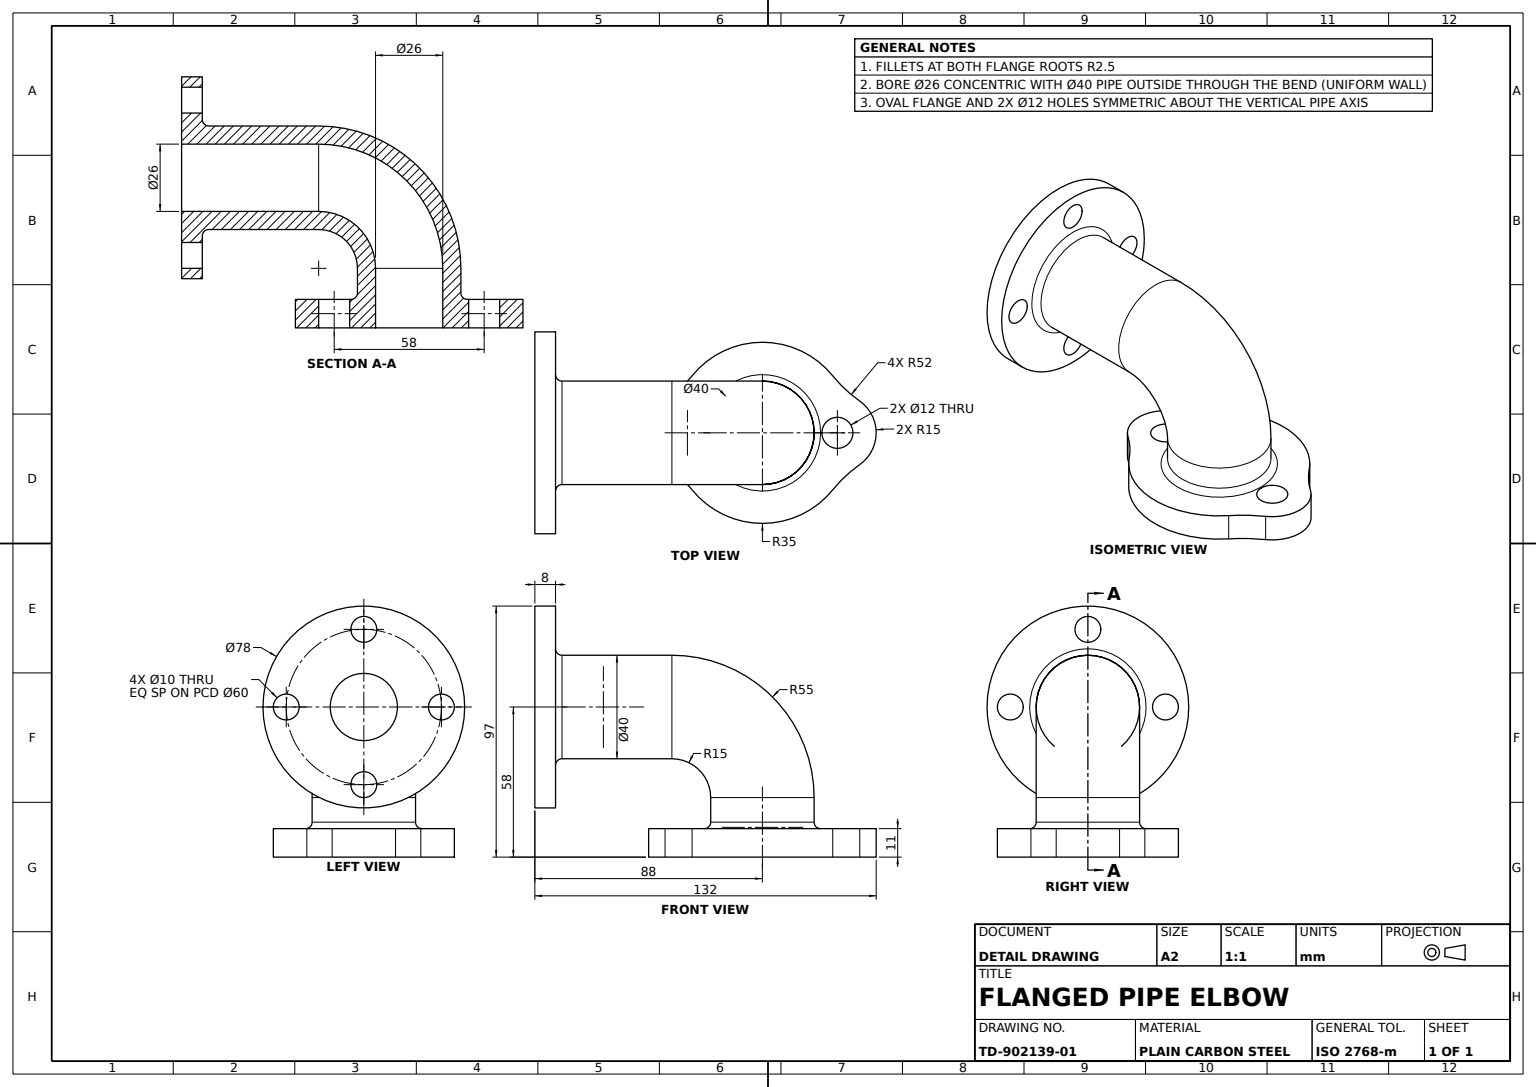
SolidWorks part; units mm, degrees
material "Plain Carbon Steel"
ref_plane "Front Plane" through (0, 0, 0) normal (0, 0, 1) x (1, 0, 0)
ref_plane "Top Plane" through (0, 0, 0) normal (0, 1, 0) x (1, 0, 0)
ref_plane "Right Plane" through (0, 0, 0) normal (1, 0, 0) x (0, 0, -1)
sketch "Elbow Path Sketch" plane through (0, 0, 0) normal (0, 0, 1) x (1, 0, 0)
  line L0 (0, 0) -> (53, 0)
  line L1 (88, -35) -> (88, -58)
  arc A0 (53, 0) -> (88, -35) centre (53, -35) cw
  dimension "D3" = 35
  dimension "D1" = 88
  dimension "D2" = 58
sketch "Pipe Section Sketch Ø40xØ26" plane through (0, 0, 0) normal (1, 0, 0) x (0, 0, -1)
  circle A0 centre (0, 0) radius 20
  circle A1 centre (0, 0) radius 13
  dimension "D1" = 40
  dimension "D2" = 26
sweep "Elbow Pipe Body" add profiles "Pipe Section Sketch Ø40xØ26" path "Elbow Path Sketch"
sketch "Round Flange Sketch Ø78" plane through (0, 0, 0) normal (1, 0, 0) x (0, 0, -1)
  circle A0 centre (0, 0) radius 39
  circle A1 centre (0, 0) radius 13 construction
  circle A2 centre (0, 0) radius 13
  dimension "D1" = 78
extrude "Round Flange Ø78" add sketch "Round Flange Sketch Ø78" along normal blind 8
sketch "Round Flange Bolt Holes Sketch" plane through (0, 0, 0) normal (-1, 0, 0) x (0, 0, 1)
  circle A0 centre (0, 30) radius 5
  circle A1 centre (0, 0) radius 30 construction
  circle A2 centre (30, 0) radius 5
  circle A3 centre (0, -30) radius 5
  circle A4 centre (-30, 0) radius 5
  point P14 (0, 0)
  dimension "D1" = 60
  dimension "D2" = 10
  dimension "D4" = 30
  dimension "D5" = 30
  dimension "D3" = 4
extrude "Round Flange Bolt Holes 4xØ10" cut sketch "Round Flange Bolt Holes Sketch" against normal up to next
sketch "Oval Flange Sketch" plane through (0, -58, 0) normal (0, -1, 0) x (1, 0, 0)
  arc A0 (60.8032, -22.0303) -> (115.1968, -22.0303) centre (88, 0) ccw
  circle A1 centre (88, 0) radius 29 construction
  circle A2 centre (117, 0) radius 6
  circle A3 centre (59, 0) radius 6
  circle A4 centre (88, 0) radius 13 construction
  circle A5 centre (88, 0) radius 13
  arc A6 (125.6426, -12.2599) -> (125.6426, 12.2599) centre (117, 0) ccw
  arc A7 (50.3574, 12.2599) -> (50.3574, -12.2599) centre (59, 0) ccw
  arc A8 (115.1968, 22.0303) -> (60.8032, 22.0303) centre (88, 0) ccw
  arc A9 (115.1968, -22.0303) -> (125.6426, -12.2599) centre (155.6034, -54.7611) cw
  arc A10 (125.6426, 12.2599) -> (115.1968, 22.0303) centre (155.6034, 54.7611) cw
  arc A11 (60.8032, 22.0303) -> (50.3574, 12.2599) centre (20.3966, 54.7611) cw
  arc A12 (60.8032, -22.0303) -> (50.3574, -12.2599) centre (20.3966, -54.7611) ccw
  dimension "D1" = 70
  dimension "D2" = 58
  dimension "D3" = 12
  dimension "D4" = 30
  dimension "D5" = 52
extrude "Oval Flange" add sketch "Oval Flange Sketch" against normal blind 11
fillet "Flange Root Fillets R2.5" radius 2.5 2 edges at (68, -47, 0) (8, 0, -20)
